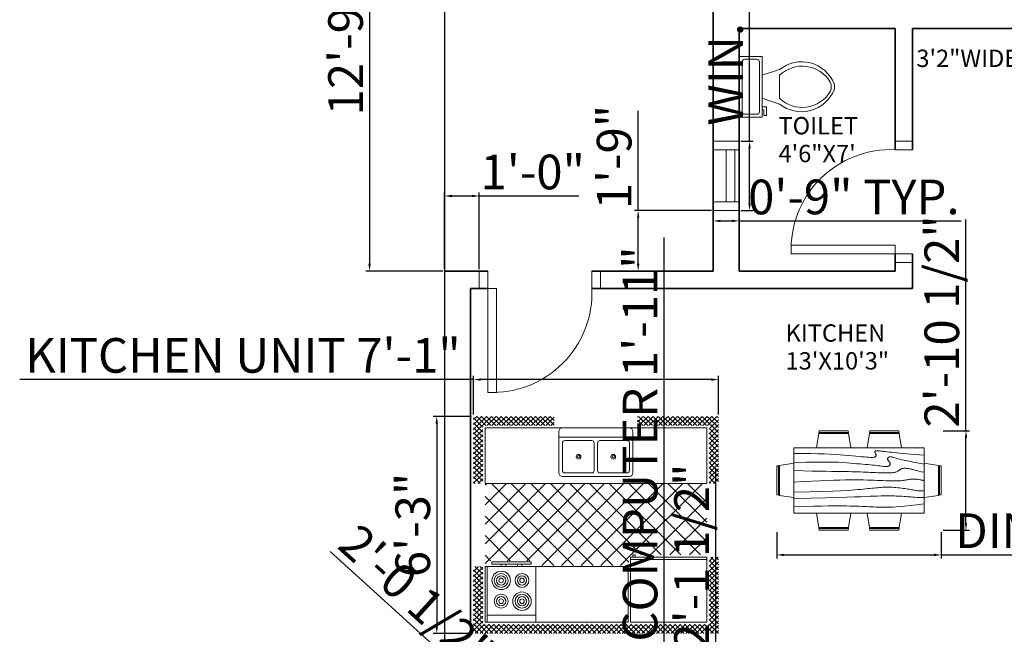
# Model space of a CAD drawing. Units: inches. Extents: x 2021 to 2692, y 429 to 1061.
# Tile 2 of 5: x 2021 to 2362, y 708 to 921. Entities that reach past the tile are written whole.
import ezdxf

# ---------------------------------------------------------------- set-up
doc = ezdxf.new("R2010")
doc.units = ezdxf.units.IN
for name, color, linetype, lineweight in [('A-ANNO-DIMS', 2, 'Continuous', 18), ('A-AREA-IDEN', 7, 'Continuous', 18), ('A-DOOR', 4, 'Continuous', 18), ('A-FLOR-FIXT', 9, 'Continuous', 18), ('A-FURN', 8, 'Continuous', 13), ('A-GLAZ', 4, 'Continuous', 18), ('A-WALL', 7, 'Continuous', 35), ('C-PROP', 3, 'Continuous', 25)]:
    doc.layers.add(name, color=color, linetype=linetype, lineweight=lineweight)
doc.styles.get("Standard").update_dxf_attribs({"font": 'arial.ttf'})
doc.dimstyles.new('ISO-25', dxfattribs={"dimtxt": 12, "dimasz": 2.5, "dimexe": 1.25, "dimexo": 0.625, "dimtad": 1, "dimdec": 0, "dimlunit": 3, "dimtxsty": 'Standard', "dimcen": 2.5, "dimadec": 0, "dimazin": 0, "dimtfac": 1, "dimtdec": 0, "dimtmove": 0, "dimatfit": 3, "dimfxl": 1, "dimarcsym": 0})

# ---------------------------------------------------------------- blocks, each defined once
blk = doc.blocks.new('Dining Set - 36 x 72 in.')
for p, q in [((-22, 27.5), (-22.1562, 26.50042)), ((-22, 27.5), (-6, 27.5)), ((-5.8437, 26.49966), (-6, 27.5)), ((6, 27.5), (5.8438, 26.50042)), ((6, 27.5), (22, 27.5)), ((22.1563, 26.49966), (22, 27.5)), ((-22.2343, 26.00059), (-23.4847, 17.99762)), ((-22.2304, 26), (-5.7608, 26)), ((-5.8416, 26.5), (-22.1534, 26.5)), ((-4.5152, 17.99762), (-5.7655, 25.99926)), ((5.7657, 26.00059), (4.5153, 17.99762)), ((5.7696, 26), (22.2392, 26)), ((22.1584, 26.5), (5.8466, 26.5)), ((23.4848, 17.99762), (22.2345, 25.99926)), ((36, 18), (-36, 18)), ((-36, 18), (-36, -18)), ((36, -18), (36, 18)), ((-45.5, 8), (-44.5004, 8.15617)), ((-45.5, 8), (-45.5, -8)), ((-44.5, -8.15843), (-44.5, 8.15338)), ((-44.0006, 8.23428), (-35.9976, 9.48474)), ((-44, 8.23041), (-44, -8.23915)), ((44.0006, 8.23428), (35.9976, 9.48474)), ((44, 8.23041), (44, -8.23915)), ((44.5, -8.15843), (44.5, 8.15338)), ((45.5, 8), (44.5005, 8.15617)), ((45.5, 8), (45.5, -8)), ((-44.4997, -8.15631), (-45.5, -8)), ((-35.9976, -9.48476), (-43.9993, -8.2345)), ((35.9976, -9.48476), (43.9993, -8.2345)), ((44.4997, -8.15631), (45.5, -8)), ((-36, -18), (36, -18)), ((-22.2343, -26.0006), (-23.4847, -17.99762)), ((-4.5152, -17.99762), (-5.7655, -25.99928)), ((5.7657, -26.0006), (4.5153, -17.99762)), ((23.4848, -17.99762), (22.2345, -25.99928)), ((-22.2304, -26), (-5.7608, -26)), ((-22, -27.5), (-22.1562, -26.50044)), ((-5.8416, -26.5), (-22.1534, -26.5)), ((-5.8437, -26.49967), (-6, -27.5)), ((5.7696, -26), (22.2392, -26)), ((6, -27.5), (5.8438, -26.50044)), ((22.1584, -26.5), (5.8466, -26.5)), ((22.1563, -26.49967), (22, -27.5)), ((-22, -27.5), (-6, -27.5)), ((6, -27.5), (22, -27.5))]:
    blk.add_line(p, q)
for points in [[(-36, 15), (-31.1772, 14.97754), (-26.8079, 14.91406), (-22.8538, 14.81543), (-19.276, 14.6875), (-16.0362, 14.53613), (-13.0957, 14.36718), (-10.4159, 14.18652), (-7.9583, 14), (-5.6904, 13.81315), (-3.6035, 13.63021), (-1.6954, 13.45508), (0.0365, 13.29166), (1.5945, 13.14388), (2.9811, 13.01562), (4.1988, 12.9108), (5.25, 12.83333), (6.1393, 12.78613), (6.8802, 12.76823), (7.4883, 12.77767), (7.9792, 12.8125), (8.3685, 12.87077), (8.6719, 12.95052), (8.9049, 13.0498), (9.0833, 13.16666), (9.2205, 13.29899), (9.3216, 13.44401), (9.3895, 13.59879), (9.4271, 13.76041), (9.4373, 13.92594), (9.4232, 14.09245), (9.3875, 14.257), (9.3333, 14.41666), (9.2638, 14.56917), (9.1836, 14.71484), (9.0975, 14.85465), (9.0104, 14.98958), (8.9272, 15.1206), (8.8529, 15.2487), (8.7922, 15.37483), (8.75, 15.5), (8.7305, 15.62467), (8.7344, 15.74739), (8.7617, 15.86621), (8.8125, 15.97916), (8.8867, 16.08431), (8.9844, 16.17968), (9.1055, 16.26334), (9.25, 16.33333), (9.4189, 16.38802), (9.6172, 16.42708), (9.8506, 16.45052), (10.125, 16.45833), (10.4463, 16.45052), (10.8203, 16.42708), (11.2529, 16.38802), (11.75, 16.33333), (12.3184, 16.26318), (12.9694, 16.17838), (13.7151, 16.07991), (14.5677, 15.96875), (15.5395, 15.84586), (16.6426, 15.71224), (17.8893, 15.56884), (19.2917, 15.41666), (20.859, 15.25667), (22.5879, 15.08984), (24.4721, 14.91715), (26.5052, 14.73958), (28.6809, 14.5581), (30.9929, 14.3737), (33.4347, 14.18733), (36, 14)], [(-36, 10), (-28.9766, 10.14274), (-23.1725, 10.20442), (-18.4241, 10.19775), (-14.5677, 10.13541), (-11.4399, 10.03011), (-8.877, 9.89453), (-6.7154, 9.74137), (-4.7917, 9.58333), (-2.9698, 9.43082), (-1.2246, 9.28515), (0.4415, 9.14534), (2.026, 9.01041), (3.5266, 8.87939), (4.9408, 8.7513), (6.266, 8.62516), (7.5, 8.5), (8.6411, 8.37549), (9.6914, 8.2539), (10.6538, 8.13818), (11.5312, 8.03125), (12.3267, 7.93603), (13.043, 7.85547), (13.6831, 7.79248), (14.25, 7.75), (14.7471, 7.7303), (15.1797, 7.73307), (15.5537, 7.75732), (15.875, 7.80208), (16.1494, 7.86637), (16.3828, 7.94922), (16.5811, 8.04964), (16.75, 8.16666), (16.8944, 8.29915), (17.0143, 8.44531), (17.1089, 8.60319), (17.1771, 8.77083), (17.218, 8.94629), (17.2305, 9.1276), (17.2137, 9.31282), (17.1667, 9.5), (17.0895, 9.6875), (16.987, 9.875), (16.8649, 10.0625), (16.7292, 10.25), (16.5856, 10.4375), (16.4401, 10.625), (16.2985, 10.8125), (16.1667, 11), (16.05, 11.18733), (15.9518, 11.3737), (15.8752, 11.5581), (15.8229, 11.73958), (15.798, 11.91715), (15.8034, 12.08984), (15.842, 12.25667), (15.9167, 12.41666), (16.0295, 12.56836), (16.1784, 12.70833), (16.3605, 12.83268), (16.5729, 12.9375), (16.8127, 13.01888), (17.0768, 13.07291), (17.3625, 13.0957), (17.6667, 13.08333), (17.9894, 13.03312), (18.3418, 12.94726), (18.7382, 12.82918), (19.1927, 12.68229), (19.7195, 12.51001), (20.3327, 12.31575), (21.0465, 12.10294), (21.875, 11.875), (22.8357, 11.63354), (23.959, 11.37304), (25.2786, 11.08618), (26.8282, 10.76562), (28.6414, 10.40405), (30.752, 9.99414), (33.1936, 9.52856), (36, 9)], [(-36, 5.5), (-30.7157, 5.3348), (-26.069, 5.20963), (-21.9946, 5.11767), (-18.4271, 5.05208), (-15.3009, 5.00602), (-12.5508, 4.97265), (-10.1112, 4.94515), (-7.9167, 4.91666), (-5.909, 4.88167), (-4.0586, 4.83984), (-2.3429, 4.79215), (-0.7396, 4.73958), (0.7739, 4.6831), (2.22, 4.6237), (3.6213, 4.56233), (5, 4.5), (6.373, 4.43782), (7.7344, 4.3776), (9.0723, 4.32129), (10.375, 4.27083), (11.6309, 4.22819), (12.8281, 4.19531), (13.9551, 4.17415), (15, 4.16666), (15.954, 4.17448), (16.819, 4.19791), (17.6001, 4.23698), (18.3021, 4.29166), (18.9299, 4.36198), (19.4883, 4.44791), (19.9823, 4.54948), (20.4167, 4.66666), (20.7969, 4.79899), (21.1302, 4.94401), (21.4245, 5.09879), (21.6875, 5.26041), (21.9271, 5.42594), (22.1511, 5.59245), (22.3672, 5.757), (22.5834, 5.91666), (22.8065, 6.06868), (23.0404, 6.21093), (23.2879, 6.34147), (23.5521, 6.45833), (23.8358, 6.55957), (24.142, 6.64323), (24.4735, 6.70735), (24.8334, 6.75), (25.2235, 6.76969), (25.642, 6.76692), (26.0858, 6.74267), (26.5521, 6.69791), (27.0379, 6.63362), (27.5404, 6.55078), (28.0565, 6.45036), (28.5834, 6.33333), (29.1242, 6.19987), (29.7071, 6.04687), (30.3661, 5.87044), (31.1354, 5.66666), (32.0493, 5.43164), (33.142, 5.16146), (34.4475, 4.85221), (36, 4.5)], [(-36, -1), (-30.7915, -0.6591), (-26.0195, -0.38216), (-21.6519, -0.16284), (-17.6563, 0.00521), (-14.0005, 0.12833), (-10.6523, 0.21289), (-7.5796, 0.26522), (-4.75, 0.29166), (-2.134, 0.29793), (0.2878, 0.28711), (2.5317, 0.26163), (4.6146, 0.22396), (6.5529, 0.17651), (8.3633, 0.12174), (10.0623, 0.06209), (11.6667, 0), (13.1899, -0.06201), (14.6341, -0.1211), (15.9982, -0.17432), (17.2813, -0.21875), (18.4823, -0.25147), (19.6003, -0.26953), (20.6343, -0.27002), (21.5834, -0.25), (22.4481, -0.20768), (23.2357, -0.14584), (23.9549, -0.06836), (24.6146, 0.02083), (25.2235, 0.11784), (25.7904, 0.21875), (26.3241, 0.31966), (26.8334, 0.41666), (27.3265, 0.50618), (27.8099, 0.58593), (28.2894, 0.65397), (28.7709, 0.70833), (29.2601, 0.74707), (29.763, 0.76823), (30.2855, 0.76985), (30.8334, 0.75), (31.4088, 0.70784), (31.9994, 0.64713), (32.589, 0.57275), (33.1615, 0.48958), (33.7008, 0.4025), (34.1908, 0.3164), (34.6153, 0.23616), (34.9584, 0.16666), (35.2099, 0.11165), (35.3848, 0.07031), (35.504, 0.04069), (35.5886, 0.02083), (35.6594, 0.00879), (35.7377, 0.0026), (35.8442, 0.00032), (36, 0)], [(-36, -6.5), (-27.1843, -6.31267), (-20.084, -6.1263), (-14.469, -5.9419), (-10.1094, -5.76042), (-6.7752, -5.58285), (-4.2363, -5.41016), (-2.2629, -5.24333), (-0.625, -5.08334), (0.8708, -4.93099), (2.2715, -4.78646), (3.5872, -4.64974), (4.8281, -4.52084), (6.0046, -4.39974), (7.127, -4.28646), (8.2053, -4.18099), (9.25, -4.08334), (10.2705, -3.99382), (11.2734, -3.91407), (12.2647, -3.84603), (13.25, -3.79167), (14.2354, -3.75293), (15.2266, -3.73177), (16.2295, -3.73015), (17.25, -3.75), (18.2912, -3.79248), (19.3451, -3.85547), (20.4009, -3.93604), (21.4479, -4.03125), (22.4754, -4.13819), (23.4727, -4.25391), (24.4289, -4.37549), (25.3334, -4.5), (26.1785, -4.62492), (26.9694, -4.74935), (27.7145, -4.87281), (28.4219, -4.99479), (29.1, -5.11483), (29.7572, -5.23242), (30.4016, -5.34709), (31.0417, -5.45834), (31.6837, -5.56437), (32.3262, -5.65821), (32.9658, -5.73153), (33.599, -5.77604), (34.2224, -5.78345), (34.8327, -5.74545), (35.4264, -5.65373), (36, -5.5)], [(-36, -10), (-26.4022, -9.81299), (-18.4675, -9.62891), (-11.9839, -9.45069), (-6.7396, -9.28125), (-2.5226, -9.12354), (0.8789, -8.98047), (3.6769, -8.85498), (6.0833, -8.75), (8.2767, -8.66765), (10.3021, -8.60677), (12.1712, -8.56543), (13.8958, -8.54167), (15.4876, -8.53353), (16.9583, -8.53907), (18.3197, -8.55632), (19.5834, -8.58334), (20.7616, -8.61841), (21.8685, -8.66081), (22.9188, -8.71004), (23.9271, -8.76563), (24.9081, -8.82707), (25.8763, -8.89388), (26.8465, -8.96558), (27.8334, -9.04167), (28.8474, -9.12118), (29.8828, -9.20117), (30.93, -9.27824), (31.9792, -9.34896), (33.0205, -9.40991), (34.0443, -9.45768), (35.0407, -9.48885), (36, -9.5)], [(-36, -14.5), (-30.0881, -14.33513), (-25.0332, -14.21224), (-20.7312, -14.12647), (-17.0781, -14.07292), (-13.97, -14.04671), (-11.3027, -14.04297), (-8.9724, -14.05681), (-6.875, -14.08334), (-4.9224, -14.11833), (-3.0905, -14.16016), (-1.3709, -14.20785), (0.2448, -14.26042), (1.7647, -14.3169), (3.1973, -14.3763), (4.5507, -14.43767), (5.8333, -14.5), (7.0554, -14.5621), (8.235, -14.62175), (9.3922, -14.67652), (10.5469, -14.72396), (11.7192, -14.76164), (12.929, -14.78711), (14.1965, -14.79794), (15.5417, -14.79167), (16.9933, -14.76424), (18.6152, -14.70508), (20.4804, -14.60197), (22.6615, -14.44271), (25.2312, -14.21509), (28.2624, -13.9069), (31.8277, -13.50594), (36, -13)]]:
    blk.add_lwpolyline(points)
blk = doc.blocks.new('Kitchen Layout - 7 x 8 ft')
for p, q in [((-5, 81.32), (2.68, 89)), ((-5, 83.44), (0.56, 89)), ((-5, 85.56), (-1.56, 89)), ((-5, 87.68), (-3.68, 89)), ((-1, 84.97), (-5, 88.97)), ((-1, 82.85), (-5, 86.85)), ((1.09, 85), (-2.91, 89)), ((3.21, 85), (-0.79, 89)), ((0.81, 85), (4.81, 89)), ((5.34, 85), (1.34, 89)), ((2.93, 85), (6.93, 89)), ((7.46, 85), (3.46, 89)), ((5.05, 85), (9.05, 89)), ((9.58, 85), (5.58, 89)), ((7.17, 85), (11.17, 89)), ((11.7, 85), (7.7, 89)), ((9.29, 85), (13.29, 89)), ((13.82, 85), (9.82, 89)), ((11.41, 85), (15.41, 89)), ((15.94, 85), (11.94, 89)), ((13.53, 85), (17.53, 89)), ((18.06, 85), (14.06, 89)), ((15.65, 85), (19.65, 89)), ((20.18, 85), (16.18, 89)), ((17.78, 85), (21.78, 89)), ((22.31, 85), (18.31, 89)), ((19.9, 85), (23.9, 89)), ((24.43, 85), (20.43, 89)), ((22.02, 85), (26.02, 89)), ((26.55, 85), (22.55, 89)), ((24.14, 85), (28.14, 89)), ((28.67, 85), (24.67, 89)), ((26.26, 85), (30.26, 89)), ((30.79, 85), (26.79, 89)), ((28.38, 85), (32.38, 89)), ((32.91, 85), (28.91, 89)), ((30.5, 85), (34.5, 89)), ((35.03, 85), (31.03, 89)), ((32.63, 85), (36.63, 89)), ((37.16, 85), (33.16, 89)), ((34.75, 85), (38.75, 89)), ((39.28, 85), (35.28, 89)), ((36.87, 85), (40.87, 89)), ((41.4, 85), (37.4, 89)), ((38.99, 85), (42.99, 89)), ((43.52, 85), (39.52, 89)), ((41.11, 85), (45.11, 89)), ((45.64, 85), (41.64, 89)), ((43.23, 85), (47.23, 89)), ((47.76, 85), (43.76, 89)), ((45.35, 85), (49.35, 89)), ((49.88, 85), (45.88, 89)), ((47.47, 85), (51.47, 89)), ((52, 85), (48, 89)), ((49.6, 85), (53.6, 89)), ((54.13, 85), (50.13, 89)), ((51.72, 85), (55.72, 89)), ((56.25, 85), (52.25, 89)), ((53.84, 85), (57.84, 89)), ((58.37, 85), (54.37, 89)), ((55.96, 85), (59.96, 89)), ((60.49, 85), (56.49, 89)), ((58.08, 85), (62.08, 89)), ((62.61, 85), (58.61, 89)), ((60.2, 85), (64.2, 89)), ((64.73, 85), (60.73, 89)), ((62.32, 85), (66.32, 89)), ((66.85, 85), (62.85, 89)), ((64.45, 85), (68.45, 89)), ((68.97, 85), (64.97, 89)), ((66.57, 85), (70.57, 89)), ((71.1, 85), (67.1, 89)), ((68.69, 85), (72.69, 89)), ((73.22, 85), (69.22, 89)), ((70.81, 85), (74.81, 89)), ((75.34, 85), (71.34, 89)), ((72.93, 85), (76.93, 89)), ((77.46, 85), (73.46, 89)), ((75.05, 85), (79.05, 89)), ((79.58, 85), (75.58, 89)), ((77.17, 85), (81.17, 89)), ((81.7, 85), (77.7, 89)), ((79.29, 85), (83.29, 89)), ((83.82, 85), (79.82, 89)), ((81.42, 85), (85.42, 89)), ((85.95, 85), (81.95, 89)), ((83.54, 85), (87.54, 89)), ((88.07, 85), (84.07, 89)), ((85.66, 85), (89.66, 89)), ((90.19, 85), (86.19, 89)), ((87.78, 85), (91.78, 89)), ((92.31, 85), (88.31, 89)), ((89.9, 85), (93.9, 89)), ((94.43, 85), (90.43, 89)), ((92.02, 85), (96.02, 89)), ((96.55, 85), (92.55, 89)), ((94.14, 85), (98.14, 89)), ((101, 82.67), (94.67, 89)), ((96.27, 85), (100.27, 89)), ((101, 84.79), (96.79, 89)), ((97, 83.61), (101, 87.61)), ((97, 81.49), (101, 85.49)), ((101, 86.92), (98.92, 89)), ((-1, 80.73), (-5, 84.73)), ((-5, 79.19), (-1, 83.19)), ((-1, 78.61), (-5, 82.61)), ((-5, 77.07), (-1, 81.07)), ((34, 84), (96, 84)), ((34, 60), (34, 84)), ((74, 81), (95, 81)), ((96, 84), (96, 60)), ((101, 80.55), (97, 84.55)), ((97, 79.37), (101, 83.37)), ((101, 78.43), (97, 82.43)), ((97, 77.25), (101, 81.25)), ((-1, 76.49), (-5, 80.49)), ((-5, 74.95), (-1, 78.95)), ((-1, 74.36), (-5, 78.36)), ((-5, 72.83), (-1, 76.83)), ((101, 76.31), (97, 80.31)), ((97, 75.13), (101, 79.13)), ((101, 74.19), (97, 78.19)), ((97, 73.01), (101, 77.01)), ((-1, 72.24), (-5, 76.24)), ((-5, 70.71), (-1, 74.71)), ((-1, 70.12), (-5, 74.12)), ((-5, 68.59), (-1, 72.59)), ((101, 72.07), (97, 76.07)), ((97, 70.89), (101, 74.89)), ((101, 69.95), (97, 73.95)), ((97, 68.76), (101, 72.76)), ((-1, 68), (-5, 72)), ((-5, 66.47), (-1, 70.47)), ((-1, 65.88), (-5, 69.88)), ((-5, 64.35), (-1, 68.35)), ((101, 67.82), (97, 71.82)), ((97, 66.64), (101, 70.64)), ((101, 65.7), (97, 69.7)), ((97, 64.52), (101, 68.52)), ((-1, 63.76), (-5, 67.76)), ((-5, 62.22), (-1, 66.22)), ((-1, 61.64), (-5, 65.64)), ((-5, 60.1), (-1, 64.1)), ((101, 63.58), (97, 67.58)), ((97, 62.4), (101, 66.4)), ((101, 61.46), (97, 65.46)), ((97, 60.28), (101, 64.28)), ((-1, 59.52), (-5, 63.52)), ((-5, 57.98), (-1, 61.98)), ((-1, 57.39), (-5, 61.39)), ((-4.86, 56), (-1, 59.86)), ((96, 60), (34, 60)), ((80, 60), (80, 59)), ((82, 59), (82, 60)), ((87, 59), (87, 60)), ((89, 60), (89, 59)), ((100.34, 60), (97, 63.34)), ((98.22, 60), (97, 61.22)), ((98.84, 60), (101, 62.16)), ((100.96, 60), (101, 60.04)), ((-1.73, 56), (-5, 59.27)), ((-3.85, 56), (-5, 57.15)), ((-2.74, 56), (-1, 57.74)), ((0, 57), (33, 57)), ((10.4, 24), (45.9, 59.5)), ((18.88, 24), (54.38, 59.5)), ((27.37, 24), (62.87, 59.5)), ((31, 55), (31, 56)), ((32, 56), (32, 55)), ((33.03, 55.11), (37.41, 59.5)), ((67.71, 24), (33.68, 58.04)), ((35.85, 24), (71.35, 59.5)), ((76.2, 24), (40.7, 59.5)), ((44.34, 24), (77.84, 57.5)), ((84.68, 24), (49.18, 59.5)), ((52.82, 24), (86.32, 57.5)), ((93.17, 24), (57.67, 59.5)), ((61.31, 24), (96, 58.69)), ((96, 29.65), (66.15, 59.5)), ((96, 38.14), (76.64, 57.5)), ((96, 46.63), (85.13, 57.5)), ((96, 55.11), (93.57, 57.54)), ((0, 30.57), (24.43, 55)), ((0, 39.06), (15.94, 55)), ((0, 47.54), (7.46, 55)), ((1.91, 24), (32.91, 55)), ((33.77, 24), (2.77, 55)), ((42.26, 24), (11.26, 55)), ((50.74, 24), (19.74, 55)), ((59.23, 24), (28.23, 55)), ((32, 55), (31, 55)), ((25.29, 24), (0, 49.29)), ((69.79, 24), (96, 50.21)), ((16.8, 24), (0, 40.8)), ((78.28, 24), (96, 41.72)), ((8.32, 24), (0, 32.32)), ((86.76, 24), (96, 33.24)), ((-5, 21.92), (-2.92, 24)), ((-5, 19.8), (-1, 23.8)), ((-1, 19.21), (-5, 23.21)), ((-5, 17.68), (-1, 21.68)), ((-1, 21.33), (-3.67, 24)), ((-1, 23.45), (-1.55, 24)), ((0, 24), (96, 24)), ((0, 0), (0, 24)), ((95.25, 24), (96, 24.75)), ((96, 24), (96, 0)), ((97, 22.1), (98.9, 24)), ((97, 19.97), (101, 23.97)), ((101, 19.03), (97, 23.03)), ((97, 17.85), (101, 21.85)), ((101, 21.16), (98.16, 24)), ((101, 23.28), (100.28, 24)), ((-1, 17.09), (-5, 21.09)), ((-5, 15.55), (-1, 19.55)), ((-1, 14.97), (-5, 18.97)), ((-5, 13.43), (-1, 17.43)), ((47.25, 6.5), (47.25, 18.5)), ((48.75, 18.5), (48.75, 6.5)), ((101, 16.91), (97, 20.91)), ((97, 15.73), (101, 19.73)), ((101, 14.79), (97, 18.79)), ((97, 13.61), (101, 17.61)), ((-1, 12.85), (-5, 16.85)), ((-5, 11.31), (-1, 15.31)), ((-1, 10.73), (-5, 14.73)), ((-5, 9.19), (-1, 13.19)), ((101, 12.67), (97, 16.67)), ((97, 11.49), (101, 15.49)), ((101, 10.55), (97, 14.55)), ((97, 9.37), (101, 13.37)), ((-1, 8.6), (-5, 12.6)), ((-5, 7.07), (-1, 11.07)), ((-1, 6.48), (-5, 10.48)), ((-5, 4.95), (-1, 8.95)), ((101, 8.43), (97, 12.43)), ((97, 7.25), (101, 11.25)), ((101, 6.31), (97, 10.31)), ((97, 5.12), (101, 9.12)), ((-1, 4.36), (-5, 8.36)), ((-5, 2.83), (-1, 6.83)), ((-1, 2.24), (-5, 6.24)), ((-5, 0.71), (-1, 4.71)), ((101, 4.18), (97, 8.18)), ((97, 3), (101, 7)), ((101, 2.06), (97, 6.06)), ((97, 0.88), (101, 4.88)), ((-1, 0.12), (-5, 4.12)), ((-5, -1.42), (-1, 2.58)), ((2, -5), (-5, 2)), ((-5, -3.54), (-1, 0.46)), ((96, 0), (0, 0)), ((64, 4), (32, 4)), ((93.24, -5), (101, 2.76)), ((95.36, -5), (101, 0.64)), ((101, -0.06), (97, 3.94)), ((101, -2.18), (97, 1.82)), ((-0.12, -5), (-5, -0.12)), ((-2.25, -5), (-5, -2.25)), ((-4.34, -5), (-0.34, -1)), ((-2.22, -5), (1.78, -1)), ((-0.1, -5), (3.9, -1)), ((4.12, -5), (0.12, -1)), ((2.02, -5), (6.02, -1)), ((6.24, -5), (2.24, -1)), ((4.14, -5), (8.14, -1)), ((8.36, -5), (4.36, -1)), ((6.27, -5), (10.27, -1)), ((10.48, -5), (6.48, -1)), ((8.39, -5), (12.39, -1)), ((12.6, -5), (8.6, -1)), ((10.51, -5), (14.51, -1)), ((14.73, -5), (10.73, -1)), ((12.63, -5), (16.63, -1)), ((16.85, -5), (12.85, -1)), ((14.75, -5), (18.75, -1)), ((18.97, -5), (14.97, -1)), ((16.87, -5), (20.87, -1)), ((21.09, -5), (17.09, -1)), ((18.99, -5), (22.99, -1)), ((23.21, -5), (19.21, -1)), ((21.11, -5), (25.11, -1)), ((25.33, -5), (21.33, -1)), ((23.24, -5), (27.24, -1)), ((27.45, -5), (23.45, -1)), ((25.36, -5), (29.36, -1)), ((29.57, -5), (25.57, -1)), ((27.48, -5), (30, -2.48)), ((30, -3.3), (27.7, -1)), ((30, -1.18), (29.82, -1)), ((66, -2.54), (67.54, -1)), ((66, -4.66), (69.66, -1)), ((69.88, -5), (66, -1.12)), ((67.76, -5), (66, -3.24)), ((67.78, -5), (71.78, -1)), ((72, -5), (68, -1)), ((69.9, -5), (73.9, -1)), ((74.12, -5), (70.12, -1)), ((72.03, -5), (76.03, -1)), ((76.24, -5), (72.24, -1)), ((74.15, -5), (78.15, -1)), ((78.36, -5), (74.36, -1)), ((76.27, -5), (80.27, -1)), ((80.49, -5), (76.49, -1)), ((78.39, -5), (82.39, -1)), ((82.61, -5), (78.61, -1)), ((80.51, -5), (84.51, -1)), ((84.73, -5), (80.73, -1)), ((82.63, -5), (86.63, -1)), ((86.85, -5), (82.85, -1)), ((84.75, -5), (88.75, -1)), ((88.97, -5), (84.97, -1)), ((86.88, -5), (90.88, -1)), ((91.09, -5), (87.09, -1)), ((89, -5), (93, -1)), ((93.21, -5), (89.21, -1)), ((91.12, -5), (95.12, -1)), ((95.34, -5), (91.34, -1)), ((97.46, -5), (93.46, -1)), ((99.58, -5), (95.58, -1)), ((101, -4.3), (97, -0.3)), ((97.48, -5), (101, -1.48)), ((99.6, -5), (101, -3.6)), ((-4.37, -5), (-5, -4.37)), ((29.6, -5), (30, -4.6))]:
    blk.add_line(p, q)
for points in [[(0, 56), (0, 84), (33, 84), (33, 56)], [(74, 60), (74, 84), (95, 84), (95, 60)], [(76, 58), (76, 59), (93, 59), (93, 58)]]:
    blk.add_lwpolyline(points, close=True)
for points in [[(32, 1.5), (32, 19.5)], [(33.5, 21), (62.5, 21)], [(33.5, 6.5), (33.5, 18.5)], [(34.5, 19.5), (46.25, 19.5)], [(49.75, 19.5), (61.5, 19.5)], [(62.5, 18.5), (62.5, 6.5)], [(64, 19.5), (64, 1.5)], [(46.25, 5.5), (34.5, 5.5)], [(61.5, 5.5), (49.75, 5.5)], [(62.5, 0), (33.5, 0)]]:
    blk.add_lwpolyline(points)
for centre, radius in [((80, 75), 4), ((80, 75), 3), ((80, 75), 2), ((89, 75), 3), ((89, 75), 2), ((80, 75), 1), ((89, 75), 1), ((80, 66), 3), ((89, 66), 4), ((89, 66), 3), ((80, 66), 2), ((80, 66), 1), ((89, 66), 2), ((89, 66), 1), ((40.5, 12.5), 1), ((40.5, 12.5), 0.5), ((55.5, 12.5), 1), ((55.5, 12.5), 0.5)]:
    blk.add_circle(centre, radius)
for centre, radius, start, end in [((33.5, 19.5), 1.5, 90, 180), ((34.5, 18.5), 1, 90, 180), ((46.25, 18.5), 1, 0, 90), ((49.75, 18.5), 1, 90, 180), ((61.5, 18.5), 1, 0, 90), ((62.5, 19.5), 1.5, 0, 90), ((34.5, 6.5), 1, 180, 270), ((46.25, 6.5), 1, 270, 0), ((49.75, 6.5), 1, 180, 270), ((61.5, 6.5), 1, 270, 0), ((33.5, 1.5), 1.5, 180, 270), ((62.5, 1.5), 1.5, 270, 0)]:
    blk.add_arc(centre, radius, start, end)
blk = doc.blocks.new('Toilet - top')
for p, q in [((9.5, -6), (9.5, -2)), ((-10, -8.5), (-8, -8.5)), ((-10, -9.5), (-10, -8.5)), ((-7, -9.5), (-10, -9.5)), ((-8, -8.5), (-8, -8)), ((-7, -8), (-7, -9.5)), ((-4, -8), (-6, -14)), ((4, -8), (6, -14)), ((4, -14), (-4, -14))]:
    blk.add_line(p, q)
blk.add_lwpolyline([(10.5, -8), (10.5, 0), (-10.5, 0), (-10.5, -8)], close=True)
for points in [[(-9.5, -2), (-9.5, -6)], [(8.5, -1), (-8.5, -1)], [(-8.5, -7), (8.5, -7)]]:
    blk.add_lwpolyline(points)
for centre, radius, start, end in [((-8.62, -1.88), 0.884, 81.8699, 188.1301), ((8.62, -1.88), 0.884, 351.8699, 98.1301), ((-8.62, -6.12), 0.884, 171.8699, 278.1301), ((8.62, -6.12), 0.884, 261.8699, 8.1301), ((3.52, -21.58), 12.17, 141.4691, 247.9714), ((4.2, -21.82), 11.33, 136.3677, 238.9468), ((-3.52, -21.58), 12.17, 292.0284, 38.5307), ((-4.2, -21.82), 11.33, 301.053, 43.6321), ((0, -27.88), 4, 245.7318, 294.2682), ((0, -29), 4, 254.8605, 285.1395)]:
    blk.add_arc(centre, radius, start, end)
blk = doc.blocks.new('DOOR-SWING-36IN')
for p, q in [((36.03, 42), (42.03, 42)), ((36.03, 39), (42.03, 39)), ((36.03, 3), (42.03, 3)), ((36.03, 0), (42.03, 0))]:
    blk.add_line(p, q)
blk.add_lwpolyline([(36.03, 39), (0.03, 39), (0.03, 36), (36.03, 36)], close=True)
blk.add_arc((34.53, 37.5), 34.53, 177.5104, 272.4896)
blk = doc.blocks.new('WIN-18IN')
for p, q in [((9, 24), (0, 24)), ((0, 21), (0, 3)), ((9, 21), (0, 21)), ((4.5, 21), (4.5, 3)), ((7.5, 21), (7.5, 3)), ((9, 3), (9, 21)), ((0, 3), (9, 3)), ((0, 0), (9, 0))]:
    blk.add_line(p, q)
blk = doc.blocks.new('*D23')
at = {"layer": 'A-ANNO-DIMS', "color": 0, "lineweight": -2, "transparency": 16777216}
for p, q in [((2206.25, 666.27), (2128.52, 736.94)), ((2203.95, 663.73), (2207.09, 667.19)), ((2222.48, 651.51), (2208.1, 664.59)), ((2222.03, 647.3), (2225.17, 650.75))]:
    blk.add_line(p, q, dxfattribs=at)
at = {"layer": 'A-ANNO-DIMS', "color": 0, "transparency": 16777216}
for points in [[(2208.38, 664.89), (2207.82, 664.28), (2206.25, 666.27)], [(2222.76, 651.82), (2222.2, 651.2), (2224.33, 649.83)]]:
    blk.add_solid(points, dxfattribs=at)
at = {"layer": 'Defpoints', "color": 0, "transparency": 16777216}
for p in [(2206.25, 666.27), (2203.53, 663.27), (2221.61, 646.83)]:
    blk.add_point(p, dxfattribs=at)
at = {"layer": 'A-ANNO-DIMS', "color": 0, "transparency": 16777216, "insert": (2171.05, 707.5), "char_height": 12, "attachment_point": 5, "rotation": 317.7243}
blk.add_mtext('2\'-0 1/2" TYP.', dxfattribs=at)
blk = doc.blocks.new('*D34')
at = {"layer": 'A-ANNO-DIMS', "color": 0, "lineweight": -2, "transparency": 16777216}
for p, q in [((2270.11, 938.55), (2270.11, 932.96)), ((2303.16, 938.55), (2303.16, 932.96)), ((2270.11, 934.21), (2160.14, 934.21)), ((2300.66, 934.21), (2272.61, 934.21))]:
    blk.add_line(p, q, dxfattribs=at)
at = {"layer": 'A-ANNO-DIMS', "color": 0, "transparency": 16777216}
for points in [[(2272.61, 934.63), (2272.61, 933.8), (2270.11, 934.21)], [(2300.66, 934.63), (2300.66, 933.8), (2303.16, 934.21)]]:
    blk.add_solid(points, dxfattribs=at)
at = {"layer": 'Defpoints', "color": 0, "transparency": 16777216}
for p in [(2270.11, 939.17), (2303.16, 939.17), (2270.11, 934.21)]:
    blk.add_point(p, dxfattribs=at)
at = {"layer": 'A-ANNO-DIMS', "color": 0, "transparency": 16777216, "insert": (2213.87, 941.04), "char_height": 12, "attachment_point": 5}
blk.add_mtext('WC 2\'-9" TYP.', dxfattribs=at)
blk = doc.blocks.new('*D36')
at = {"layer": 'A-ANNO-DIMS', "color": 0, "lineweight": -2, "transparency": 16777216}
for p, q in [((2273.71, 878.91), (2273.71, 1014.03)), ((2270.73, 878.91), (2274.96, 878.91)), ((2273.71, 857.41), (2273.71, 876.41)), ((2270.73, 854.91), (2274.96, 854.91))]:
    blk.add_line(p, q, dxfattribs=at)
at = {"layer": 'A-ANNO-DIMS', "color": 0, "transparency": 16777216}
for points in [[(2273.29, 876.41), (2274.13, 876.41), (2273.71, 878.91)], [(2273.29, 857.41), (2274.13, 857.41), (2273.71, 854.91)]]:
    blk.add_solid(points, dxfattribs=at)
at = {"layer": 'Defpoints', "color": 0, "transparency": 16777216}
for p in [(2270.11, 878.91), (2273.71, 878.91), (2270.11, 854.91)]:
    blk.add_point(p, dxfattribs=at)
at = {"layer": 'A-ANNO-DIMS', "color": 0, "transparency": 16777216, "insert": (2266.96, 947.72), "char_height": 12, "attachment_point": 5, "rotation": 90}
blk.add_mtext('WIN. B 2\'-0" TYP.', dxfattribs=at)
blk = doc.blocks.new('*D37')
at = {"layer": 'A-ANNO-DIMS', "color": 0, "lineweight": -2, "transparency": 16777216}
for p, q in [((2261.11, 854.28), (2261.11, 850.06)), ((2270.11, 854.28), (2270.11, 850.06)), ((2263.61, 851.31), (2267.61, 851.31)), ((2270.11, 851.31), (2347.01, 851.31))]:
    blk.add_line(p, q, dxfattribs=at)
at = {"layer": 'A-ANNO-DIMS', "color": 0, "transparency": 16777216}
for points in [[(2263.61, 851.72), (2263.61, 850.89), (2261.11, 851.31)], [(2267.61, 851.72), (2267.61, 850.89), (2270.11, 851.31)]]:
    blk.add_solid(points, dxfattribs=at)
at = {"layer": 'Defpoints', "color": 0, "transparency": 16777216}
for p in [(2261.11, 854.91), (2270.11, 854.91), (2270.11, 851.31)]:
    blk.add_point(p, dxfattribs=at)
at = {"layer": 'A-ANNO-DIMS', "color": 0, "transparency": 16777216, "insert": (2309.81, 858.06), "char_height": 12, "attachment_point": 5}
blk.add_mtext('0\'-9" TYP.', dxfattribs=at)
blk = doc.blocks.new('*D38')
at = {"layer": 'A-ANNO-DIMS', "color": 0, "lineweight": -2, "transparency": 16777216}
for p, q in [((2283.11, 743.62), (2283.11, 734.45)), ((2340.09, 743.62), (2340.09, 734.45)), ((2285.61, 735.7), (2337.59, 735.7)), ((2340.09, 735.7), (2475.73, 735.7))]:
    blk.add_line(p, q, dxfattribs=at)
at = {"layer": 'A-ANNO-DIMS', "color": 0, "transparency": 16777216}
for points in [[(2285.61, 736.12), (2285.61, 735.28), (2283.11, 735.7)], [(2337.59, 736.12), (2337.59, 735.28), (2340.09, 735.7)]]:
    blk.add_solid(points, dxfattribs=at)
at = {"layer": 'Defpoints', "color": 0, "transparency": 16777216}
for p in [(2283.11, 744.25), (2340.09, 744.25), (2340.09, 735.7)]:
    blk.add_point(p, dxfattribs=at)
at = {"layer": 'A-ANNO-DIMS', "color": 0, "transparency": 16777216, "insert": (2409.16, 742.53), "char_height": 12, "attachment_point": 5}
blk.add_mtext('DINING SET 4\'-9"', dxfattribs=at)
blk = doc.blocks.new('*D39')
at = {"layer": 'A-ANNO-DIMS', "color": 0, "lineweight": -2, "transparency": 16777216}
for p, q in [((2348.64, 778.69), (2348.64, 851.83)), ((2340.71, 778.69), (2349.89, 778.69)), ((2348.64, 746.75), (2348.64, 776.19)), ((2340.71, 744.25), (2349.89, 744.25))]:
    blk.add_line(p, q, dxfattribs=at)
at = {"layer": 'A-ANNO-DIMS', "color": 0, "transparency": 16777216}
for points in [[(2348.22, 776.19), (2349.05, 776.19), (2348.64, 778.69)], [(2348.22, 746.75), (2349.05, 746.75), (2348.64, 744.25)]]:
    blk.add_solid(points, dxfattribs=at)
at = {"layer": 'Defpoints', "color": 0, "transparency": 16777216}
for p in [(2340.09, 778.69), (2348.64, 778.69), (2340.09, 744.25)]:
    blk.add_point(p, dxfattribs=at)
at = {"layer": 'A-ANNO-DIMS', "color": 0, "transparency": 16777216, "insert": (2341.81, 816.51), "char_height": 12, "attachment_point": 5, "rotation": 90}
blk.add_mtext('2\'-10 1/2"', dxfattribs=at)
blk = doc.blocks.new('*D41')
at = {"layer": 'A-ANNO-DIMS', "color": 0, "lineweight": -2, "transparency": 16777216}
for p, q in [((2262.01, 701.96), (2262.01, 765.78)), ((2255.17, 701.96), (2263.26, 701.96)), ((2262.01, 678.75), (2262.01, 699.46)), ((2255.17, 676.25), (2263.26, 676.25))]:
    blk.add_line(p, q, dxfattribs=at)
at = {"layer": 'A-ANNO-DIMS', "color": 0, "transparency": 16777216}
for points in [[(2261.6, 699.46), (2262.43, 699.46), (2262.01, 701.96)], [(2261.6, 678.75), (2262.43, 678.75), (2262.01, 676.25)]]:
    blk.add_solid(points, dxfattribs=at)
at = {"layer": 'Defpoints', "color": 0, "transparency": 16777216}
for p in [(2254.55, 701.96), (2262.01, 701.96), (2254.55, 676.25)]:
    blk.add_point(p, dxfattribs=at)
at = {"layer": 'A-ANNO-DIMS', "color": 0, "transparency": 16777216, "insert": (2255.18, 735.12), "char_height": 12, "attachment_point": 5, "rotation": 90}
blk.add_mtext('2\'-1 1/2"', dxfattribs=at)
blk = doc.blocks.new('*D42')
at = {"layer": 'A-ANNO-DIMS', "color": 0, "lineweight": -2, "transparency": 16777216}
for p, q in [((2244.18, 700.13), (2244.18, 845.55)), ((2241.36, 700.13), (2245.43, 700.13)), ((2244.18, 679.63), (2244.18, 697.63)), ((2241.36, 677.13), (2245.43, 677.13))]:
    blk.add_line(p, q, dxfattribs=at)
at = {"layer": 'A-ANNO-DIMS', "color": 0, "transparency": 16777216}
for points in [[(2243.76, 697.63), (2244.6, 697.63), (2244.18, 700.13)], [(2243.76, 679.63), (2244.6, 679.63), (2244.18, 677.13)]]:
    blk.add_solid(points, dxfattribs=at)
at = {"layer": 'Defpoints', "color": 0, "transparency": 16777216}
for p in [(2240.73, 700.13), (2244.18, 700.13), (2240.73, 677.13)]:
    blk.add_point(p, dxfattribs=at)
at = {"layer": 'A-ANNO-DIMS', "color": 0, "transparency": 16777216, "insert": (2237.35, 774.09), "char_height": 12, "attachment_point": 5, "rotation": 90}
blk.add_mtext('COMPUTER 1\'-11"', dxfattribs=at)
blk = doc.blocks.new('*D50')
at = {"layer": 'A-ANNO-DIMS', "color": 0, "lineweight": -2, "transparency": 16777216}
for p, q in [((2178.1, 796.39), (2020.98, 796.39)), ((2178.1, 784.3), (2178.1, 797.64)), ((2260.39, 796.39), (2180.6, 796.39)), ((2262.89, 784.3), (2262.89, 797.64))]:
    blk.add_line(p, q, dxfattribs=at)
at = {"layer": 'A-ANNO-DIMS', "color": 0, "transparency": 16777216}
for points in [[(2180.6, 796.81), (2180.6, 795.97), (2178.1, 796.39)], [(2260.39, 796.81), (2260.39, 795.97), (2262.89, 796.39)]]:
    blk.add_solid(points, dxfattribs=at)
at = {"layer": 'Defpoints', "color": 0, "transparency": 16777216}
for p in [(2178.1, 796.39), (2178.1, 783.67), (2262.89, 783.67)]:
    blk.add_point(p, dxfattribs=at)
at = {"layer": 'A-ANNO-DIMS', "color": 0, "transparency": 16777216, "insert": (2098.29, 803.22), "char_height": 12, "attachment_point": 5}
blk.add_mtext('KITCHEN UNIT 7\'-1"', dxfattribs=at)
blk = doc.blocks.new('*D51')
at = {"layer": 'A-ANNO-DIMS', "color": 0, "lineweight": -2, "transparency": 16777216}
for p, q in [((2177.47, 783.67), (2164.13, 783.67)), ((2165.38, 781.17), (2165.38, 710.98)), ((2177.47, 708.48), (2164.13, 708.48))]:
    blk.add_line(p, q, dxfattribs=at)
at = {"layer": 'A-ANNO-DIMS', "color": 0, "transparency": 16777216}
for points in [[(2164.96, 781.17), (2165.8, 781.17), (2165.38, 783.67)], [(2164.96, 710.98), (2165.8, 710.98), (2165.38, 708.48)]]:
    blk.add_solid(points, dxfattribs=at)
at = {"layer": 'Defpoints', "color": 0, "transparency": 16777216}
for p in [(2178.1, 783.67), (2165.38, 708.48), (2178.1, 708.48)]:
    blk.add_point(p, dxfattribs=at)
at = {"layer": 'A-ANNO-DIMS', "color": 0, "transparency": 16777216, "insert": (2158.62, 746.08), "char_height": 12, "attachment_point": 5, "rotation": 90}
blk.add_mtext('6\'-3"', dxfattribs=at)
blk = doc.blocks.new('*D53')
at = {"layer": 'A-ANNO-DIMS', "color": 0, "lineweight": -2, "transparency": 16777216}
for p, q in [((2167.48, 986.96), (2140.87, 986.96)), ((2142.12, 984.46), (2142.12, 836.46)), ((2167.48, 833.96), (2140.87, 833.96))]:
    blk.add_line(p, q, dxfattribs=at)
at = {"layer": 'A-ANNO-DIMS', "color": 0, "transparency": 16777216}
for points in [[(2141.71, 984.46), (2142.54, 984.46), (2142.12, 986.96)], [(2141.71, 836.46), (2142.54, 836.46), (2142.12, 833.96)]]:
    blk.add_solid(points, dxfattribs=at)
at = {"layer": 'Defpoints', "color": 0, "transparency": 16777216}
for p in [(2168.11, 986.96), (2142.12, 833.96), (2168.11, 833.96)]:
    blk.add_point(p, dxfattribs=at)
at = {"layer": 'A-ANNO-DIMS', "color": 0, "transparency": 16777216, "insert": (2135.37, 910.46), "char_height": 12, "attachment_point": 5, "rotation": 90}
blk.add_mtext('12\'-9"', dxfattribs=at)
blk = doc.blocks.new('*D65')
at = {"layer": 'A-ANNO-DIMS', "color": 0, "lineweight": -2, "transparency": 16777216}
for p, q in [((2168.11, 834.59), (2168.11, 861.2)), ((2170.61, 859.95), (2177.61, 859.95)), ((2180.11, 834.59), (2180.11, 861.2)), ((2180.11, 859.95), (2214.63, 859.95))]:
    blk.add_line(p, q, dxfattribs=at)
at = {"layer": 'A-ANNO-DIMS', "color": 0, "transparency": 16777216}
for points in [[(2170.61, 860.37), (2170.61, 859.53), (2168.11, 859.95)], [(2177.61, 860.37), (2177.61, 859.53), (2180.11, 859.95)]]:
    blk.add_solid(points, dxfattribs=at)
at = {"layer": 'Defpoints', "color": 0, "transparency": 16777216}
for p in [(2180.11, 859.95), (2168.11, 833.96), (2180.11, 833.96)]:
    blk.add_point(p, dxfattribs=at)
at = {"layer": 'A-ANNO-DIMS', "color": 0, "transparency": 16777216, "insert": (2198.62, 866.7), "char_height": 12, "attachment_point": 5}
blk.add_mtext('1\'-0"', dxfattribs=at)
blk = doc.blocks.new('*D67')
at = {"layer": 'A-ANNO-DIMS', "color": 0, "lineweight": -2, "transparency": 16777216}
for p, q in [((2235.12, 854.91), (2235.12, 889.43)), ((2260.48, 854.91), (2233.87, 854.91)), ((2235.12, 836.46), (2235.12, 852.41)), ((2260.48, 833.96), (2233.87, 833.96))]:
    blk.add_line(p, q, dxfattribs=at)
at = {"layer": 'A-ANNO-DIMS', "color": 0, "transparency": 16777216}
for points in [[(2234.71, 852.41), (2235.54, 852.41), (2235.12, 854.91)], [(2234.71, 836.46), (2235.54, 836.46), (2235.12, 833.96)]]:
    blk.add_solid(points, dxfattribs=at)
at = {"layer": 'Defpoints', "color": 0, "transparency": 16777216}
for p in [(2235.12, 854.91), (2261.11, 854.91), (2261.11, 833.96)]:
    blk.add_point(p, dxfattribs=at)
at = {"layer": 'A-ANNO-DIMS', "color": 0, "transparency": 16777216, "insert": (2228.37, 873.42), "char_height": 12, "attachment_point": 5, "rotation": 90}
blk.add_mtext('1\'-9"', dxfattribs=at)

msp = doc.modelspace()

# ---------------------------------------------------------------- linework, layer by layer
at = {"layer": 'A-WALL'}
for p, q in [((2261.11, 833.96), (2261.11, 939.69)), ((2270.11, 833.96), (2270.11, 917.96)), ((2324.11, 917.96), (2270.11, 917.96)), ((2324.11, 875.96), (2324.11, 917.96)), ((2366.11, 917.96), (2330.11, 917.96)), ((2330.11, 875.96), (2330.11, 917.96)), ((2324.11, 833.96), (2324.11, 839.96)), ((2330.11, 833.96), (2330.11, 839.96)), ((2183.11, 833.96), (2168.11, 833.96)), ((2261.11, 833.96), (2219.11, 833.96)), ((2324.11, 833.96), (2270.11, 833.96)), ((2330.11, 833.96), (2330.11, 827.96)), ((2177.11, 827.96), (2177.11, 707.96)), ((2183.11, 827.96), (2177.11, 827.96)), ((2330.11, 827.96), (2219.11, 827.96))]:
    msp.add_line(p, q, dxfattribs=at)
at = {"layer": 'C-PROP'}
msp.add_lwpolyline([(2168.11, 506.96), (2528.11, 506.96), (2528.11, 986.96), (2168.11, 986.96)], close=True, dxfattribs=at)

# ---------------------------------------------------------------- block references
at = {"layer": 'A-DOOR', "extrusion": (0, 0, -1), "zscale": -1, "rotation": 180}
msp.add_blockref('DOOR-SWING-36IN', (-2288.08, 878.96), dxfattribs=at)
at = {"layer": 'A-DOOR', "rotation": 90.00000000000072}
msp.add_blockref('DOOR-SWING-36IN', (2222.11, 791.93), dxfattribs=at)
at = {"layer": 'A-FLOR-FIXT', "rotation": 90}
msp.add_blockref('Toilet - top', (2270.11, 897.75), dxfattribs=at)
at = {"layer": 'A-FLOR-FIXT', "xscale": 0.7999071535793756, "yscale": 0.7999071535793756, "zscale": 0.7999071535793756, "rotation": 180}
msp.add_blockref('Kitchen Layout - 7 x 8 ft', (2258.89, 779.67), dxfattribs=at)
at = {"layer": 'A-FURN', "xscale": 0.6261809615206749, "yscale": 0.6261809615206749, "zscale": 0.6261809615206749}
msp.add_blockref('Dining Set - 36 x 72 in.', (2311.6, 761.47), dxfattribs=at)
at = {"layer": 'A-GLAZ'}
msp.add_blockref('WIN-18IN', (2261.11, 854.91), dxfattribs=at)

# ---------------------------------------------------------------- texts
at = {"layer": 'A-AREA-IDEN'}
for s, p in [('3\'2"WIDE', (2331.45, 904.59)), ('TOILET', (2283.71, 881.27)), ('4\'6"X7\'', (2283.71, 871.63)), ('KITCHEN', (2286.16, 809.51)), ('13\'X10\'3"', (2286.16, 799.87))]:
    msp.add_text(s, height=6, dxfattribs=at).set_placement(p)

# ---------------------------------------------------------------- dimensions: what is measured, and where the dimension line sits
at = {"layer": 'A-ANNO-DIMS'}
for base, p1, p2, angle, text, picture, middle in [((2273.71, 878.91), (2270.11, 854.91), (2270.11, 878.91), 90, 'WIN. B <> TYP.', '*D36', (2266.96, 947.72)), ((2270.1097, 934.2138), (2303.156, 939.1708), (2270.1097, 939.1708), 180, 'WC <> TYP.', '*D34', (2213.8729, 941.0435)), ((2244.18, 700.13), (2240.73, 677.13), (2240.73, 700.13), 90, 'COMPUTER <>', '*D42', (2237.35, 774.09)), ((2178.1, 796.39), (2262.89, 783.67), (2178.1, 783.67), 180, 'KITCHEN UNIT <>', '*D50', (2098.29, 803.22)), ((2206.25, 666.27), (2221.61, 646.83), (2203.53, 663.27), 137.7243, '<> TYP.', '*D23', (2171.05, 707.5))]:
    dim = msp.add_linear_dim(base=base, p1=p1, p2=p2, angle=angle, text=text, dimstyle='ISO-25', override={"dimdec": 1, "dimlfac": 1, "dimrnd": 0, "dimzin": 1, "dimdsep": 46, "dimlunit": 4, "dimfrac": 2}, dxfattribs=at)
    dim.commit()
    dim.dimension.update_dxf_attribs({"geometry": picture, "text_midpoint": middle})
for base, p1, p2, angle, picture, middle in [((2142.12, 833.96), (2168.11, 986.96), (2168.11, 833.96), 90, '*D53', (2135.37, 910.46)), ((2235.1247, 854.9061), (2261.1097, 833.9642), (2261.1097, 854.9061), 90, '*D67', (2228.3729, 873.4159)), ((2180.11, 859.95), (2168.11, 833.96), (2180.11, 833.96), 0, '*D65', (2198.62, 866.7)), ((2348.64, 778.69), (2340.09, 744.25), (2340.09, 778.69), 90, '*D39', (2341.81, 816.51)), ((2165.38, 708.48), (2178.1, 783.67), (2178.1, 708.48), 270, '*D51', (2158.62, 746.08)), ((2262.01, 701.96), (2254.55, 676.25), (2254.55, 701.96), 90, '*D41', (2255.18, 735.12))]:
    dim = msp.add_linear_dim(base=base, p1=p1, p2=p2, angle=angle, dimstyle='ISO-25', override={"dimdec": 1, "dimlfac": 1, "dimrnd": 0, "dimzin": 1, "dimdsep": 46, "dimlunit": 4, "dimfrac": 2}, dxfattribs=at)
    dim.commit()
    dim.dimension.update_dxf_attribs({"geometry": picture, "text_midpoint": middle})
for base, p1, p2, text, picture, middle in [((2270.11, 851.31), (2261.11, 854.91), (2270.11, 854.91), '<> TYP.', '*D37', (2309.81, 858.06)), ((2340.09, 735.7), (2283.11, 744.25), (2340.09, 744.25), 'DINING SET <>', '*D38', (2409.16, 742.53))]:
    dim = msp.add_linear_dim(base=base, p1=p1, p2=p2, text=text, dimstyle='ISO-25', override={"dimdec": 1, "dimlfac": 1, "dimrnd": 0, "dimzin": 1, "dimdsep": 46, "dimlunit": 4, "dimfrac": 2}, dxfattribs=at)
    dim.commit()
    dim.dimension.update_dxf_attribs({"geometry": picture, "text_midpoint": middle})

doc.saveas('drawing.dxf')
